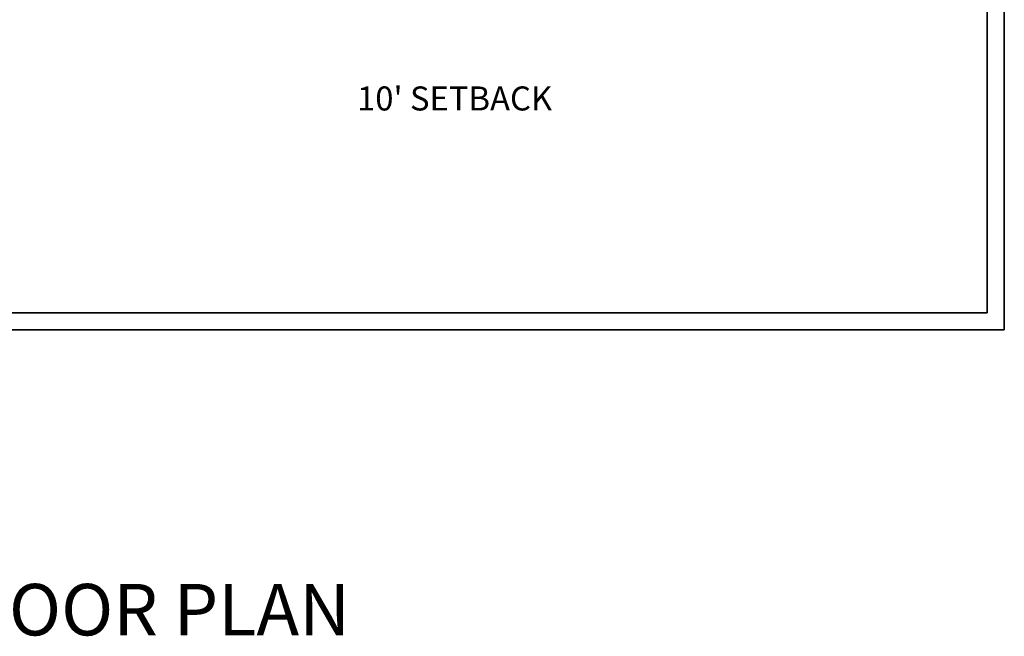
# Model space of a CAD drawing. Units: inches. Extents: x 3008 to 4088, y 1255 to 2137.
# Tile 22 of 30: x 3796 to 4083, y 1260 to 1440. Entities that reach past the tile are written whole.
import ezdxf

# ---------------------------------------------------------------- set-up
doc = ezdxf.new("R2010")
doc.units = ezdxf.units.IN
doc.layers.add('A-ANNO-TEXT', color=7, linetype='Continuous', lineweight=18)
doc.layers.add('C-PROP', color=1, linetype='Continuous', lineweight=35)
doc.styles.get("Standard").update_dxf_attribs({"font": 'arial.ttf'})

msp = doc.modelspace()

# ---------------------------------------------------------------- linework, layer by layer
at = {"layer": 'C-PROP'}
for p, q in [((4082.94, 2009.72), (4082.94, 1349.72)), ((4077.94, 2004.72), (4077.94, 1354.72)), ((4077.94, 1354.72), (3607.94, 1354.72)), ((4082.94, 1349.72), (3602.94, 1349.72))]:
    msp.add_line(p, q, dxfattribs=at)

# ---------------------------------------------------------------- texts
at = {"layer": 'A-ANNO-TEXT', "attachment_point": 1}
for s, width, insert, char_height in [("{\\fTimes New Roman|b0|i0|c0|p18;10' SETBACK}", 105.6127, (3894.56, 1420.66), 7), ('{\\fTimes New Roman|b0|i0|c0|p18;FIRST FLOOR PLAN}', 294.0396, (3711.51, 1275.76), 15)]:
    msp.add_mtext_dynamic_manual_height_columns(s, width=width, gutter_width=12.5, heights=[0], dxfattribs=dict(at, insert=insert, char_height=char_height))

doc.saveas('drawing.dxf')
